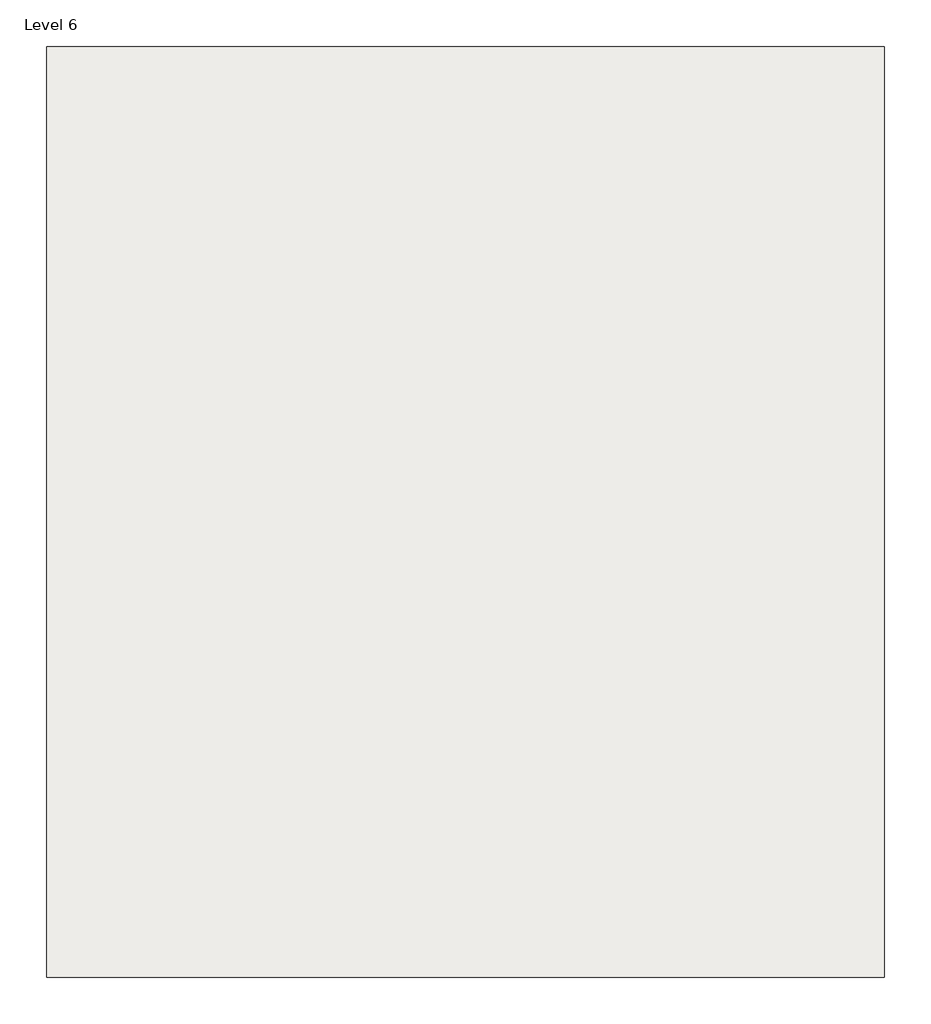
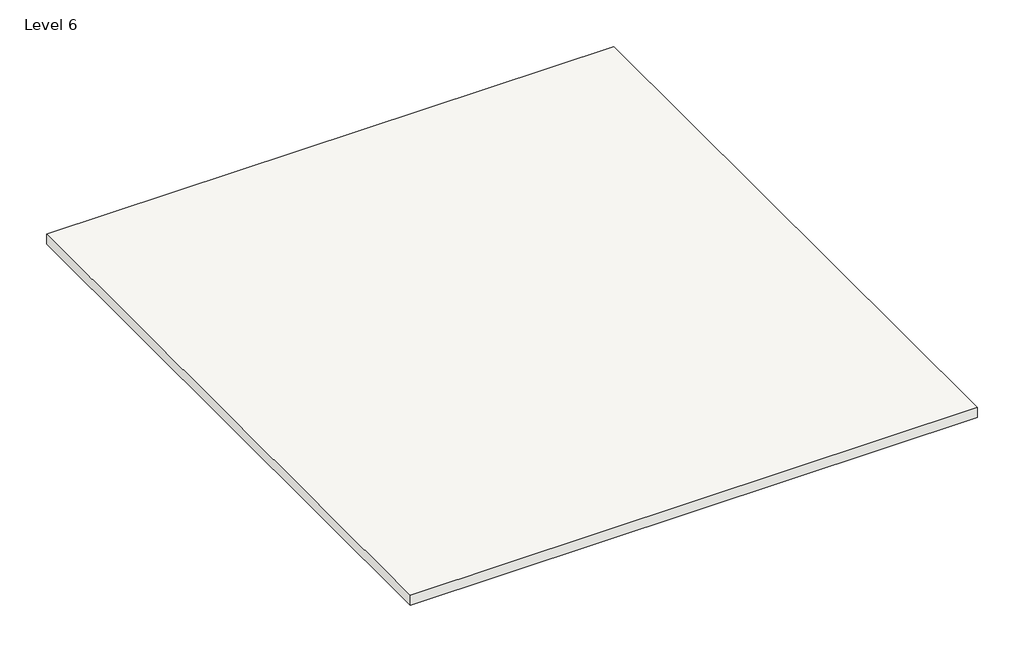
# One storey: 1 roof.
"""IFC4 building model written with IfcOpenShell, lengths in millimetres."""

from ifc_helpers import new_model, si_unit, frame, origin, place, context, project, spatial, polyline, outline, extrude, element, save

model = new_model("IFC4")

# Units and contexts
model_context = context("Model", 3, world=origin())
ifc_project = project(units=[si_unit("LENGTHUNIT", "METRE", prefix="MILLI")], contexts=[model_context])

# Site, building, storey
site = spatial("IfcSite", under=ifc_project)
building = spatial("IfcBuilding", under=site)
storey = spatial("IfcBuildingStorey", under=building, Name="Level 6", Elevation=15240.0)

# Roof
placement = place(None, origin())
element("IfcRoof", 1, ObjectType="Generic - 12\"", at=placement, inside=storey, context=model_context, shape_type="SweptSolid", body=[
    extrude(outline(polyline([(1270.0, 14776.9372886), (9499.6, 14776.9372886), (9499.6, 5632.9372886), (1270.0, 5632.9372886), (1270.0, 14776.9372886)])), frame((0.0, 0.0, 15240.0), z_axis=(0.0, 0.0, 1.0), x_axis=(1.0, 0.0, 0.0)), (0.0, 0.0, 1.0), 152.4),
])

save(model, "model.ifc")

# Revit data of these elements
# Type "Generic - 12\""
#   Assembly Code = "B1020"
#   Layers, outside or top first: 0' - 6" no material (function 1)
# Element 1 (IfcRoof, "Generic - 12\"")
#   built-in parameter 1001705 = 50.5 (stored number, unit not read)
#   built-in parameter 1001710 = 33615
#   Phase Created = New Construction
#   Materials on its faces: "Clad - White", "Default Roof"
# Materials
#   "Clad - White": class "Wood", colour RGB 242 242 238, transparency 0, Cost = 0
#   "Default Roof": colour RGB 88 101 114, transparency 0, Cost = 0
